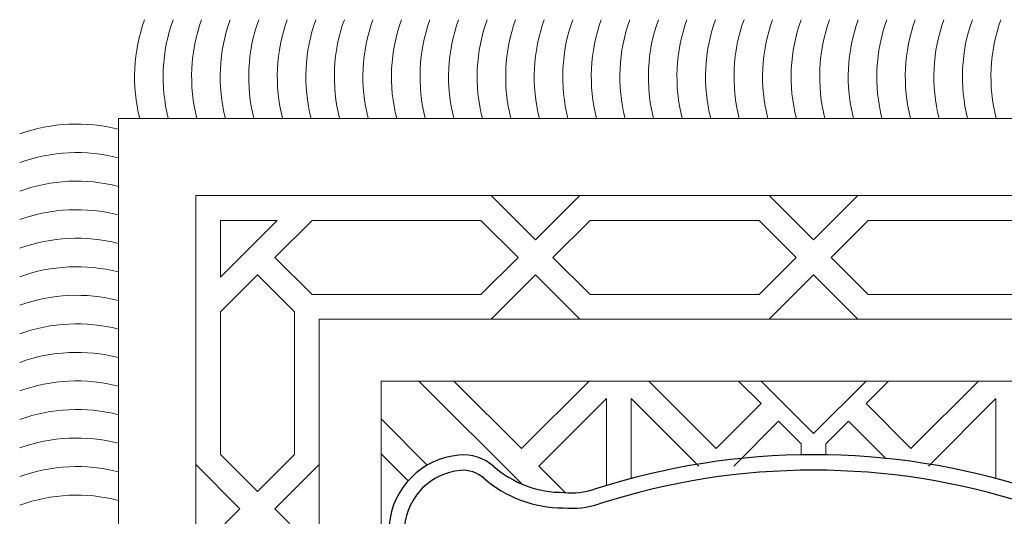
# Model space of a CAD drawing. Units: inches. Extents: x 3592 to 4861, y 1650 to 2243.
# Tile 8 of 30: x 4188.22 to 4207.34, y 1949.57 to 1959.22. Entities that reach past the tile are written whole.
import ezdxf

# ---------------------------------------------------------------- set-up
doc = ezdxf.new("R2010")
doc.units = ezdxf.units.IN
doc.layers.add('A-FURN', color=9, linetype='Continuous', lineweight=13)
doc.layers.add('RA-AP-01$0$INT', color=35, linetype='Continuous', lineweight=5)
for name, color, linetype in [('RA-AP-01$0$FURN', 3, 'Continuous'), ('RA-AP-01$0$WOOD', 64, 'Continuous'), ('RA-AP-02$0$FLPT', 30, 'Continuous')]:
    doc.layers.add(name, color=color, linetype=linetype)

# ---------------------------------------------------------------- blocks, each defined once
blk = doc.blocks.new('A$C67D63ADA')
at = {"layer": 'RA-AP-01$0$INT'}
for p, q in [((4.237240000008252, -6.353816270320467), (4.237240000008252, -6.933016270323148)), ((4.237240000008253, -6.353816270322416), (4.237240000008253, -6.933016270318608)), ((4.277240000006364, -6.923416270324413), (4.277240000021174, -6.363416270332882)), ((4.173240000008255, -6.608102561821608), (4.173240000008253, -6.498729978818613)), ((4.221240000008257, -6.608102561821311), (4.221240000008254, -6.498729978818907)), ((4.340347667501897, -6.525357395822863), (4.288553708515926, -6.525357395821494)), ((4.288553708515926, -6.525357395821494), (4.332269437266721, -6.569073124574231)), ((4.277240000015057, -6.59484772782809), (4.277240000016594, -6.536671104320128)), ((4.277240000016594, -6.536671104320128), (4.320955728767484, -6.580386833072967)), ((4.320955728767484, -6.580386833072966), (4.291867417012733, -6.609475144826422)), ((4.277240000015056, -6.59484772782809), (4.291867417012733, -6.609475144826423)), ((4.291867417012733, -6.609475144826422), (4.277240000015094, -6.594847727828128)), ((4.327336547797006, -6.596633431041195), (4.303181125511469, -6.62078885332566)), ((4.173240000008255, -6.608102561821608), (4.197240000007798, -6.632102561821458)), ((4.221240000008257, -6.608102561821311), (4.197240000007798, -6.632102561821458)), ((4.277240000014767, -6.609475144825973), (4.277240000012874, -6.677357395819498)), ((4.311181125510964, -6.64341627032368), (4.277240000014767, -6.609475144825973)), ((4.157240000008255, -6.614729978819518), (4.185926291508883, -6.643416270320512)), ((4.237240000008253, -6.614729978819338), (4.20855370850671, -6.643416270320512)), ((4.317808542507872, -6.635416270323993), (4.303181125510193, -6.620788853325663)), ((4.317808542509147, -6.635416270323988), (4.325022993004827, -6.635416270324118)), ((4.157240000008255, -6.672102561821508), (4.185926291508883, -6.643416270320512)), ((4.237240000008253, -6.672102561821688), (4.20855370850671, -6.643416270320512)), ((4.311181125510964, -6.64341627032368), (4.277240000012874, -6.677357395819498)), ((4.317808542507269, -6.65141627032399), (4.303181125510463, -6.666043687319815)), ((4.317808542508791, -6.651416270322137), (4.325022993004908, -6.651416270322329)), ((4.173240000008255, -6.678729978819417), (4.197240000007798, -6.654729978819569)), ((4.221240000008257, -6.678729978819714), (4.197240000007798, -6.654729978819569)), ((4.332269437263918, -6.695131999074563), (4.303181125510463, -6.666043687319815)), ((4.173240000008255, -6.678729978819417), (4.173240000008253, -6.788102561822412)), ((4.221240000008257, -6.678729978819714), (4.221240000008254, -6.788102561822118)), ((4.277240000012894, -6.691984812817247), (4.291867417011224, -6.677357395819567)), ((4.320955728764681, -6.706445707574319), (4.291867417011224, -6.677357395819569)), ((4.277240000012896, -6.691984812817247), (4.277240000011847, -6.750161436325209)), ((4.277240000011847, -6.750161436325209), (4.320955728764681, -6.706445707574317)), ((4.288553708510673, -6.761475144824349), (4.332269437263414, -6.717759416073553)), ((4.340347667503585, -6.761475144825284), (4.288553708510673, -6.761475144824349)), ((4.288553708510296, -6.777475144824348), (4.332269437260703, -6.821190873576702)), ((4.344903410718353, -6.777475144825364), (4.288553708510296, -6.777475144824348)), ((4.173240000008253, -6.788102561822412), (4.197240000007798, -6.812102561822261)), ((4.221240000008254, -6.788102561822118), (4.197240000007798, -6.812102561822261)), ((4.277240000011149, -6.788788853323175), (4.320955728761467, -6.832504582075438)), ((4.157240000008254, -6.794729978820322), (4.185926291507684, -6.823416270320118)), ((4.237240000008253, -6.794729978820141), (4.20855370850791, -6.823416270320116)), ((4.332269437260705, -6.821190873576701), (4.34933169350375, -6.804128617334414)), ((4.157240000008254, -6.852102561819913), (4.185926291507684, -6.823416270320118)), ((4.237240000008253, -6.852102561820093), (4.20855370850791, -6.823416270320116)), ((4.34401647081644, -6.832071257027641), (4.277240000009159, -6.898847727834922)), ((4.277240000009569, -6.876220310825392), (4.320955728761467, -6.832504582075438)), ((4.173240000009216, -6.85872997881686), (4.197240000007798, -6.834729978817973)), ((4.221240000009218, -6.858729978819082), (4.197240000007798, -6.834729978817973)), ((4.173240000009216, -6.85872997881686), (4.173240000009217, -6.968102561831729)), ((4.221240000009218, -6.858729978819082), (4.221240000009218, -6.96810256182067)), ((4.331724248043275, -6.893500564790679), (4.301808542509442, -6.923416270324519)), ((4.324435959507737, -6.923416270324613), (4.341921384145511, -6.905930845686842)), ((4.877240000006827, -6.923416270326986), (4.277240000006364, -6.923416270324413)), ((4.360068427135066, -6.99210256182739), (4.331382135628725, -6.963416270330275)), ((4.388754718631812, -6.963416270321417), (4.360068427135066, -6.99210256182739)), ((4.173240000009217, -6.968102561831729), (4.19724000000369, -6.99210256181848)), ((4.221240000009218, -6.96810256182067), (4.19724000000369, -6.99210256181848)), ((4.232553708510282, -6.97941627032422), (4.208553708513718, -7.003416270328507)), ((4.232553708510282, -6.97941627032422), (4.324754718627222, -6.979416270325234)), ((4.348754718637899, -7.003416270328198), (4.324754718627222, -6.979416270325234)), ((4.173240000009217, -6.990729978826057), (4.209926291520478, -7.027416270325517)), ((4.173240000009217, -6.990729978826057), (4.173240000009216, -7.027416270325517)), ((4.232553708503005, -7.027416270325517), (4.208553708513718, -7.003416270328507)), ((4.348754718637899, -7.003416270328198), (4.324754718648297, -7.027416270325517)), ((4.360068427138701, -7.014729978825361), (4.331382135641587, -7.043416270331702)), ((4.388754718643982, -7.043416270321417), (4.360068427138701, -7.014729978825361)), ((4.209926291520478, -7.027416270325517), (4.173240000009216, -7.027416270325517)), ((4.324754718648297, -7.027416270325517), (4.232553708503005, -7.027416270325517))]:
    blk.add_line(p, q, dxfattribs=at)
for points in [[(5.647240000006826, -6.243416270325369), (5.647240000006826, -7.09341627032537), (4.107240000006826, -7.093416270325372), (4.107240000006826, -6.19341627032537), (4.877240000006826, -6.19341627032537)], [(5.597240000006826, -6.243416270325369), (5.597240000006826, -7.04341627032537), (4.157240000006826, -7.043416270325372), (4.157240000006826, -6.243416270325369)], [(4.877240000006826, -6.32341627032537), (4.237240000006825, -6.32341627032537), (4.237240000006825, -6.963416270325371), (4.877240000006826, -6.963416270325371)]]:
    blk.add_lwpolyline(points, dxfattribs=at)
for centre, start, end in [((4.080280000005896, -6.419454311364566), 250.2038431288995, 284.3025426362932), ((4.080280000005988, -6.437934311361019), 250.2038431288995, 284.3025426362437), ((4.08028000000617, -6.456414311361291), 250.2038431288995, 284.3025426361451), ((4.080280000008625, -6.474894311361381), 250.2038431288995, 284.3025426348149), ((4.080280000006351, -6.493374311360381), 250.2038431288995, 284.3025426360469), ((4.080280000006533, -6.511854311362836), 250.2038431288995, 284.3025426359483), ((4.080280000006625, -6.530334311363108), 250.2038431288995, 284.3025426358987), ((4.080280000004351, -6.548814311359561), 250.2038431288995, 284.3025426371307), ((4.080280000006897, -6.567294311360925), 250.2038431288995, 284.302542635751), ((4.080280000006897, -6.585774311361197), 250.2038431288995, 284.302542635751), ((4.080280000007079, -6.604254311362561), 250.2038431288995, 284.3025426356524), ((4.080280000004896, -6.622734311365016), 250.2038431288995, 284.3025426368352), ((4.08028000000726, -6.64121431136165), 250.2038431288995, 284.3025426355542), ((4.080280000007443, -6.659694311363015), 250.2038431288995, 284.3025426354554), ((4.080280000005169, -6.678174311359649), 250.2038431288995, 284.3025426366875), ((4.080280000007625, -6.696654311362104), 250.2038431288995, 284.3025426353568), ((4.080280000007807, -6.715134311362376), 250.2038431288995, 284.3025426352582), ((4.080280000007897, -6.733614311363741), 250.2038431288995, 284.3025426352091), ((4.080280000005624, -6.752094311361465), 250.2038431288995, 284.302542636441), ((4.08028000000817, -6.770574311361556), 250.2038431288995, 284.3025426350613), ((4.080280000008261, -6.789054311361828), 250.2038431288995, 284.3025426350118), ((4.080280000005988, -6.807534311360646), 250.2038431288995, 284.3025426362437), ((4.08028000000617, -6.826014311360919), 250.2038431288995, 284.3025426361451), ((4.08028000000626, -6.844494311363374), 250.2038431288995, 284.302542636096), ((4.080280000008716, -6.862974311360009), 250.2038431288995, 284.3025426347654), ((4.080280000006533, -6.881454311360099), 250.2038431288995, 284.3025426359483), ((4.080280000006625, -6.899934311362554), 250.2038431288995, 284.3025426358987), ((4.080280000009079, -6.918414311359189), 250.2038431288995, 284.3025426345686), ((4.080280000006897, -6.936894311359279), 250.2038431288995, 284.302542635751), ((4.080280000006988, -6.955374311361734), 250.2038431288995, 284.3025426357019), ((4.080280000009444, -6.973854311358369), 250.2038431288995, 284.3025426343713), ((4.220001958960505, -7.12037627032743), 165.6974573630951, 199.7961568705686), ((4.238481958959504, -7.120376270325248), 165.6974573642774, 199.7961568705686), ((4.256961958958503, -7.120376270325248), 165.6974573642774, 199.7961568705686), ((4.275441958962233, -7.120376270326521), 165.6974573635878, 199.7961568705686), ((4.293921958961232, -7.120376270324339), 165.6974573647701, 199.7961568705686), ((4.312401958960231, -7.120376270324339), 165.6974573647701, 199.7961568705686), ((4.33088195896396, -7.120376270325611), 165.6974573640806, 199.7961568705686), ((4.349361958962959, -7.120376270324702), 165.6974573645733, 199.7961568705686), ((4.367841958959411, -7.120376270324702), 165.6974573645733, 199.7961568705686), ((4.386321958963322, -7.120376270325975), 165.6974573638838, 199.7961568705686), ((4.404801958962321, -7.120376270323792), 165.6974573650661, 199.7961568705686), ((4.42328195896132, -7.120376270323792), 165.6974573650661, 199.7961568705686), ((4.441761958965049, -7.120376270325065), 165.6974573643766, 199.7961568705686), ((4.460241958964048, -7.120376270324156), 165.6974573648693, 199.7961568705686)]:
    blk.add_arc(centre, 0.1091312342836184, start, end, dxfattribs=at)
blk = doc.blocks.new('A$C09A87C41')
at = {"layer": 'RA-AP-01$0$WOOD'}
for centre, radius, start, end in [((4.785350665835054, -6.643416270320894), 0.4603971832811766, 162.0683908477153, 197.9316091522852), ((4.785350665835053, -6.643416270320896), 0.4503971832811742, 162.0623235129388, 197.9376764867364), ((4.299593848995807, -6.800079200598755), 0.0500000000000024, 354.2979292346388, 17.35568397525274), ((4.299593848995804, -6.80007920059882), 0.0599999999999989, 354.823807839859, 17.40612704769988), ((4.281379376397683, -6.805679639555614), 0.0679700159630274, 318.7710509203537, 0.5333070513671823), ((4.281379376397698, -6.805679639555567), 0.0779700159630463, 318.7710509203204, 0.1376463011372249), ((4.355060862488946, -6.870248692786853), 0.0299999999999992, 138.7710509203567, 185.2568759942798), ((4.355060862488945, -6.870248692786852), 0.0199999999999984, 138.7710509203573, 185.2568759942818), ((4.374976741277023, -6.868416270320764), 0.0499999999998892, 185.256875994431, 264.7431240064054), ((4.374976741277008, -6.868416270320778), 0.0399999999998732, 185.2568759944501, 264.7431240064249)]:
    blk.add_arc(centre, radius, start, end, dxfattribs=at)
blk = doc.blocks.new('A$C44E37296')
at = {"layer": 'RA-AP-01$0$FURN'}
blk.add_blockref('A$C09A87C41', (-4.845317312134739, 7.43281203020814), dxfattribs=at)
at = {"layer": 'RA-AP-02$0$FLPT'}
blk.add_blockref('A$C67D63ADA', (-4.845317312134739, 7.43281203020814), dxfattribs=at)

msp = doc.modelspace()

# ---------------------------------------------------------------- block references
at = {"layer": 'A-FURN', "xscale": 29.98919001647196, "yscale": 29.98919001647196, "zscale": 29.98919001647196, "rotation": 270}
msp.add_blockref('A$C44E37296', (4179.961167173048, 1935.164417895216), dxfattribs=at)

doc.saveas('drawing.dxf')
